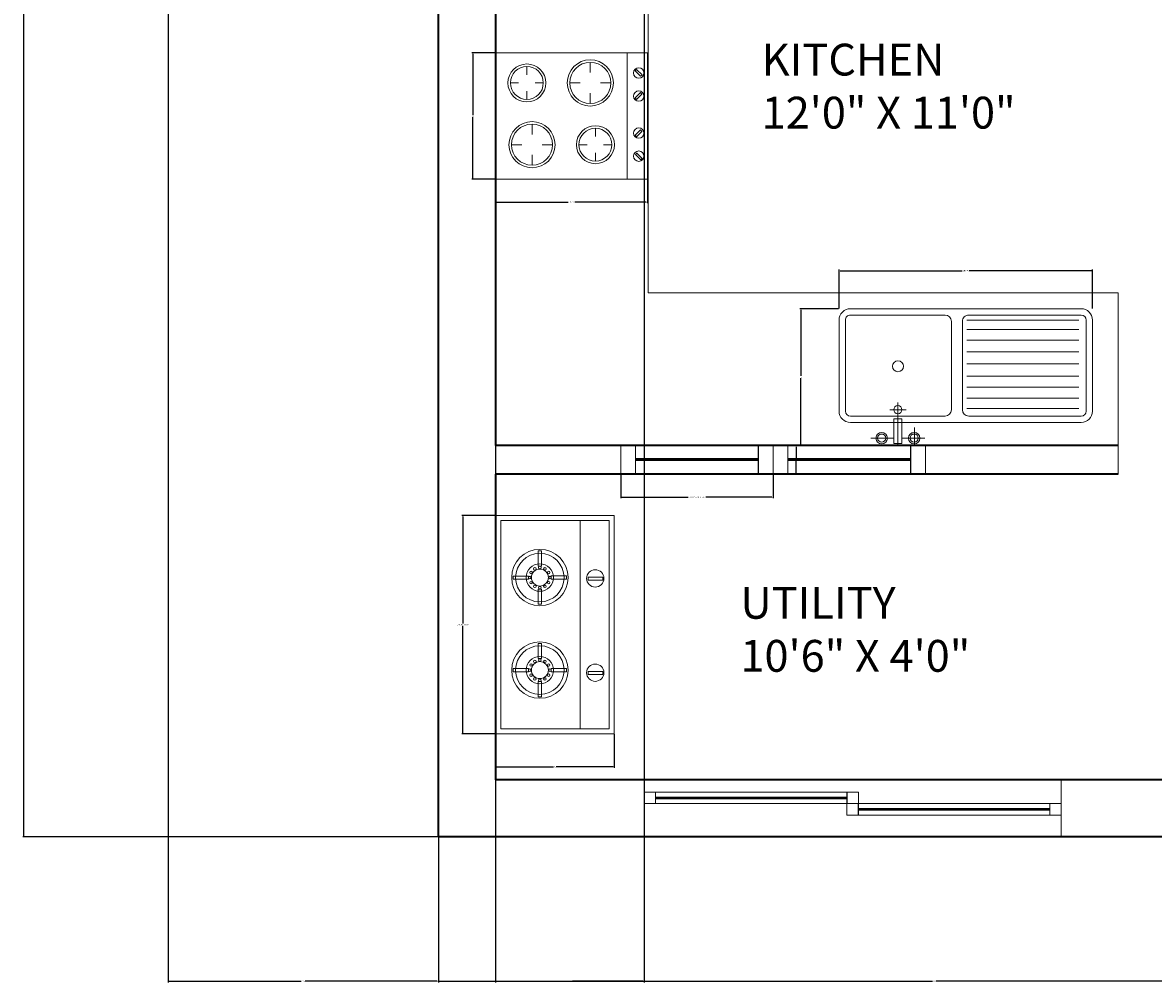
# Model space of a CAD drawing. Units: inches. Extents: x 1723 to 2209, y 1326 to 1810.
# Tile 1 of 6: x 1723 to 1901, y 1326 to 1477. Entities that reach past the tile are written whole.
import ezdxf

# ---------------------------------------------------------------- set-up
doc = ezdxf.new("R2010")
doc.units = ezdxf.units.IN
doc.layers.get('Defpoints').update_dxf_attribs({"color": 255})
for name, color, linetype, lineweight in [('A-ANNO-DIMS', 2, 'Continuous', 18), ('A-AREA-IDEN', 7, 'Continuous', 18), ('A-EQPM', 8, 'Continuous', 13), ('A-FLOR-CASE', 9, 'Continuous', 18), ('A-FLOR-FIXT', 9, 'Continuous', 18), ('A-GLAZ', 4, 'Continuous', 18), ('A-WALL', 7, 'Continuous', 35), ('Sliding Door', 3, 'Continuous', 18)]:
    doc.layers.add(name, color=color, linetype=linetype, lineweight=lineweight)
doc.styles.get("Standard").update_dxf_attribs({"font": 'arial.ttf'})
doc.dimstyles.get("Standard").update_dxf_attribs({"dimtxt": 0.18, "dimasz": 0.18, "dimexe": 0.18, "dimexo": 0.0625, "dimgap": 0.09, "dimtad": 0, "dimtih": 1, "dimtoh": 1, "dimdec": 4, "dimzin": 0, "dimdsep": 46, "dimtxsty": 'Standard', "dimcen": 0.09, "dimadec": 0, "dimazin": 0, "dimtfac": 1, "dimtdec": 4, "dimtofl": 0, "dimtmove": 0, "dimatfit": 3, "dimfxl": 1, "dimtolj": 1, "dimtzin": 0, "dimarcsym": 0})

# ---------------------------------------------------------------- blocks, each defined once
blk = doc.blocks.new('A$C01893FE0')
at = {"ltscale": 1000}
for p, q in [((705.3, 470.5), (705.3, 541.8)), ((770.8, 370.8), (770.8, 541.8)), ((754.6, 512.1), (663.9, 512.1)), ((787, 532.8), (754.6, 532.8)), ((754.6, 435.6), (754.6, 532.8)), ((787, 435.6), (787, 532.8)), ((787, 512.1), (877.6, 512.1)), ((45, 450), (958.9, 450)), ((0, 45), (0, 405)), ((25, 45), (25, 405)), ((45, 425), (490, 425)), ((583.9, 425), (958.9, 425)), ((787, 435.6), (754.6, 435.6)), ((978.9, 405), (978.9, 45)), ((1003.9, 405), (1003.9, 45)), ((53.5, 394.9), (497.4, 394.9)), ((515, 400), (515, 50)), ((558.9, 400), (558.9, 50)), ((803.2, 399.7), (738.4, 399.7)), ((53.5, 353.7), (497.4, 353.7)), ((53.5, 310.3), (497.4, 310.3)), ((53.5, 266.8), (497.4, 266.8)), ((53.5, 218.8), (497.4, 218.8)), ((53.5, 170.8), (497.4, 170.8)), ((53.5, 125), (497.4, 125)), ((53.5, 81.6), (497.4, 81.6)), ((53.5, 45), (497.4, 45)), ((490, 25), (45, 25)), ((958.9, 0), (45, 0)), ((958.9, 25), (583.9, 25))]:
    blk.add_line(p, q, dxfattribs=at)
for centre, radius in [((706.4, 512.1), 22.7), ((706.4, 512.1), 16.2), ((835.2, 512.1), 22.7), ((835.2, 512.1), 16.2), ((771.2, 399.7), 16.2), ((770.4, 227.6), 21.7)]:
    blk.add_circle(centre, radius, dxfattribs=at)
for centre, radius, start, end in [((45, 405), 45, 90, 180), ((958.9, 405), 45, 0, 90), ((45, 405), 20, 90, 180), ((490, 400), 25, 0, 90), ((583.9, 400), 25, 90, 180), ((958.9, 405), 20, 0, 90), ((45, 45), 45, 180, 270), ((45, 45), 20, 180, 270), ((490, 50), 25, 270, 0), ((583.9, 50), 25, 180, 270), ((958.9, 45), 45, 270, 0), ((958.9, 45), 20, 270, 0)]:
    blk.add_arc(centre, radius, start, end, dxfattribs=at)
blk = doc.blocks.new('A$C06E242FC')
for p, q in [((0, 455.6), (0.5, 456.1)), ((0, 455.6), (0, 0.5)), ((838.9, 456.1), (0.5, 456.1)), ((20, 435.6), (20.5, 436.1)), ((20, 435.6), (20, 20.5)), ((818.9, 436.1), (20.5, 436.1)), ((819.4, 435.6), (818.9, 436.1)), ((819.4, 20.5), (819.4, 435.6)), ((838.9, 456.1), (839.4, 455.6)), ((839.4, 0.5), (839.4, 455.6)), ((237.3, 411.5), (237.3, 356.2)), ((248.9, 411.5), (237.3, 411.5)), ((248.9, 356.2), (248.9, 411.5)), ((599.3, 411.5), (610.9, 411.5)), ((599.3, 411.5), (599.3, 356.2)), ((610.9, 356.2), (610.9, 411.5)), ((237.3, 356.2), (248.9, 356.2)), ((599.3, 356.2), (610.9, 356.2)), ((20, 324.4), (819.4, 324.4)), ((232.7, 272.7), (232.7, 214)), ((244.9, 272.7), (232.7, 272.7)), ((244.9, 214), (244.9, 272.7)), ((588.1, 272.7), (588.1, 214)), ((600.3, 272.7), (588.1, 272.7)), ((600.3, 214), (600.3, 272.7)), ((136.3, 176), (136.3, 163.8)), ((194.9, 176), (136.3, 176)), ((194.9, 163.8), (194.9, 176)), ((232.7, 214), (244.9, 214)), ((282.9, 176.3), (282.9, 164.1)), ((341.6, 176.3), (282.9, 176.3)), ((341.6, 164.1), (341.6, 176.3)), ((550.3, 176), (491.7, 176)), ((491.7, 176), (491.7, 163.8)), ((550.3, 163.8), (550.3, 176)), ((588.1, 214), (600.3, 214)), ((638.3, 176.3), (638.3, 164.1)), ((697, 176.3), (638.3, 176.3)), ((697, 164.1), (697, 176.3)), ((136.3, 163.8), (194.9, 163.8)), ((282.9, 164.1), (341.6, 164.1)), ((491.7, 163.8), (550.3, 163.8)), ((638.3, 164.1), (697, 164.1)), ((245.2, 126.1), (233, 126.1)), ((233, 126.1), (233, 67.4)), ((245.2, 67.4), (245.2, 126.1)), ((600.6, 126.1), (588.3, 126.1)), ((588.3, 126.1), (588.3, 67.4)), ((600.6, 67.4), (600.6, 126.1)), ((233, 67.4), (245.2, 67.4)), ((588.3, 67.4), (600.6, 67.4)), ((0, 0.5), (0.5, 0)), ((20, 20.5), (20.5, 20)), ((20.5, 20), (818.9, 20)), ((818.9, 20), (819.4, 20.5)), ((838.9, 0), (839.4, 0.5)), ((0.5, 0), (838.9, 0))]:
    blk.add_line(p, q)
for centre, radius in [((242, 382.9), 33.3), ((604.1, 382.9), 33.3), ((238.9, 170.1), 108.3), ((238.9, 170.1), 93.3), ((594.3, 170.1), 108.3), ((594.3, 170.1), 93.3), ((238.9, 170.1), 52.6), ((594.3, 170.1), 52.6), ((200.1, 170.1), 4.84), ((205.3, 189.5), 4.84), ((238.9, 170.1), 32.6), ((219.5, 203.7), 4.84), ((238.9, 208.9), 4.84), ((258.4, 203.7), 4.84), ((272.6, 189.5), 4.84), ((277.8, 170.1), 4.84), ((555.5, 170.1), 4.84), ((560.7, 189.5), 4.84), ((594.3, 170.1), 32.6), ((574.9, 203.7), 4.84), ((594.3, 208.9), 4.84), ((613.7, 203.7), 4.84), ((628, 189.5), 4.84), ((633.2, 170.1), 4.84), ((205.3, 150.6), 4.84), ((219.5, 136.4), 4.84), ((238.9, 131.2), 4.84), ((258.4, 136.4), 4.84), ((272.6, 150.6), 4.84), ((560.7, 150.6), 4.84), ((574.9, 136.4), 4.84), ((594.3, 131.2), 4.84), ((613.7, 136.4), 4.84), ((628, 150.6), 4.84)]:
    blk.add_circle(centre, radius)
blk = doc.blocks.new('A$C16A60262')
at = {"linetype": 'ByBlock'}
for p, q in [((0, 600), (0, 0)), ((487.7, 600), (0, 600)), ((0, 600), (500, 600)), ((0, 600), (500, 600)), ((500, 600), (500, 0)), ((500, 600), (500, 0)), ((500, 520.4), (0, 520.4)), ((119.4, 455.6), (119.4, 414.9)), ((363.3, 459.6), (363.3, 427.1)), ((38.1, 374.3), (78.8, 374.3)), ((200.7, 374.3), (160.1, 374.3)), ((298.2, 394.6), (330.7, 394.6)), ((363.3, 329.6), (363.3, 362.1)), ((428.3, 394.6), (395.8, 394.6)), ((119.4, 293), (119.4, 333.7)), ((363.3, 225.2), (363.3, 184.6)), ((119.4, 188.6), (119.4, 156.1)), ((282, 143.9), (322.6, 143.9)), ((444.5, 143.9), (403.9, 143.9)), ((54.4, 123.6), (86.9, 123.6)), ((119.4, 58.6), (119.4, 91.1)), ((184.4, 123.6), (151.9, 123.6)), ((363.3, 62.6), (363.3, 103.3)), ((0, 0), (500, 0))]:
    blk.add_line(p, q, dxfattribs=at)
for p, q in [((66.2, 557.5), (87.4, 578.7)), ((71.9, 551.8), (66.2, 557.5)), ((93.1, 573), (71.9, 551.8)), ((87.4, 578.7), (93.1, 573)), ((157.6, 572.5), (163.3, 578.1)), ((178.8, 551.2), (157.6, 572.5)), ((163.3, 578.1), (184.5, 556.9)), ((184.5, 556.9), (178.8, 551.2)), ((305.1, 572.5), (310.8, 578.1)), ((326.3, 551.2), (305.1, 572.5)), ((310.8, 578.1), (332, 556.9)), ((332, 556.9), (326.3, 551.2)), ((396.2, 558.5), (417.4, 579.7)), ((401.9, 552.8), (396.2, 558.5)), ((423.1, 574), (401.9, 552.8)), ((417.4, 579.7), (423.1, 574))]:
    blk.add_line(p, q)
for centre in [(80.1, 565.7), (171.2, 565.7), (317.6, 565.7), (408.7, 565.7)]:
    blk.add_circle(centre, 20.6)
for centre, radius in [((119.4, 374.3), 91.3), ((119.4, 374.3), 81.3), ((363.3, 394.6), 75), ((363.3, 394.6), 65), ((363.3, 143.9), 91.3), ((363.3, 143.9), 81.3), ((119.4, 123.6), 75), ((119.4, 123.6), 65)]:
    blk.add_circle(centre, radius, dxfattribs=at)
blk = doc.blocks.new('A$C7a76cbd6')
at = {"layer": 'Sliding Door'}
for p, q in [((540.4, 283.7, 0), (478.3, 283.7, 0)), ((478.3, 283.7, 0), (540.4, 283.7, 0)), ((540.4, 221.5, 0), (540.4, 283.7, 0)), ((540.4, 283.7, 0), (1585.3, 283.7, 0)), ((540.4, 283.7, 0), (540.4, 221.5, 0)), ((1585.3, 256.6, 0), (540.4, 256.6, 0)), ((540.4, 256.6, 0), (540.4, 248.7, 0)), ((540.4, 252.6, 0), (1584.3, 252.6, 0)), ((540.4, 248.7, 0), (1585.3, 248.7, 0)), ((1584.3, 283.7, 0), (1647.4, 283.7, 0)), ((1584.3, 283.7, 0), (1584.3, 221.5, 0)), ((1647.4, 283.7, 0), (1585.3, 283.7, 0)), ((1585.3, 283.7, 0), (1585.3, 221.5, 0)), ((1585.3, 248.7, 0), (1585.3, 256.6, 0)), ((1647.4, 221.5, 0), (1647.4, 283.7, 0)), ((1647.4, 283.7, 0), (1647.4, 221.5, 0)), ((478.3, 221.5, 0), (540.4, 221.5, 0)), ((478.3, 221.5, 0), (540.4, 221.5, 0)), ((1584.3, 221.5, 0), (540.4, 221.5, 0)), ((1646.4, 221.5, 0), (1584.3, 221.5, 0)), ((1584.3, 221.5, 0), (1584.3, 159.4, 0)), ((1584.3, 221.5, 0), (1647.4, 221.5, 0)), ((1584.3, 221.5, 0), (1647.4, 221.5, 0)), ((1584.3, 221.5, 0), (1584.3, 159.4, 0)), ((1585.3, 221.5, 0), (1647.4, 221.5, 0)), ((1646.4, 159.4, 0), (1646.4, 221.5, 0)), ((1647.4, 221.5, 0), (2691.3, 221.5, 0)), ((1647.4, 221.5, 0), (1647.4, 159.4, 0)), ((2691.3, 194.4, 0), (1647.4, 194.4, 0)), ((1647.4, 194.4, 0), (1647.4, 186.5, 0)), ((1647.4, 190.5, 0), (2690.3, 190.5, 0)), ((1647.4, 186.5, 0), (2691.3, 186.5, 0)), ((2690.3, 221.5, 0), (2753.4, 221.5, 0)), ((2690.3, 221.5, 0), (2690.3, 159.4, 0)), ((2753.4, 221.5, 0), (2691.3, 221.5, 0)), ((2691.3, 221.5, 0), (2691.3, 159.4, 0)), ((2691.3, 186.5, 0), (2691.3, 194.4, 0)), ((1584.3, 159.4, 0), (1646.4, 159.4, 0)), ((1584.3, 159.4, 0), (1647.4, 159.4, 0)), ((2691.3, 159.4, 0), (1646.4, 159.4, 0)), ((2690.3, 159.4, 0), (2753.4, 159.4, 0)), ((2691.3, 159.4, 0), (2753.4, 159.4, 0))]:
    blk.add_line(p, q, dxfattribs=at)
blk = doc.blocks.new('WINDOW-UTILITY-SASH')
for p, q in [((0, 4.5), (0, 0)), ((0, 4.5), (0, 0)), ((0, 4.5), (2.33, 4.5)), ((2.3, 0), (2.3, 4.5)), ((23.95, 4.5), (2.3, 4.5)), ((2.33, 4.5), (2.33, 0)), ((21.62, 4.5), (21.62, 0)), ((21.62, 4.5), (23.95, 4.5)), ((21.66, 4.5), (21.66, 0)), ((23.95, 4.5), (23.95, 0)), ((21.62, 2.47), (2.33, 2.47)), ((2.33, 2.33), (21.62, 2.33)), ((2.33, 2.18), (21.62, 2.18)), ((0, 0), (2.3, 0)), ((0, 0), (2.33, 0)), ((23.95, 0), (2.3, 0)), ((2.33, 1.29), (2.33, 1)), ((21.62, 0), (23.95, 0)), ((21.66, 1), (21.66, 1.29)), ((21.66, 0), (23.95, 0))]:
    blk.add_line(p, q)
blk = doc.blocks.new('*D77')
at = {"layer": 'A-ANNO-DIMS', "color": 0, "lineweight": -2, "transparency": 16777216}
for p, q in [((1816.79, 1405.63), (1816.79, 1401.92)), ((1840.74, 1405.63), (1840.74, 1401.92)), ((1816.97, 1402.1), (1827.36, 1402.1)), ((1840.56, 1402.1), (1830.17, 1402.1))]:
    blk.add_line(p, q, dxfattribs=at)
at = {"layer": 'A-ANNO-DIMS', "color": 0, "transparency": 16777216}
for points in [[(1816.97, 1402.13), (1816.97, 1402.07), (1816.79, 1402.1)], [(1840.56, 1402.13), (1840.56, 1402.07), (1840.74, 1402.1)]]:
    blk.add_solid(points, dxfattribs=at)
at = {"layer": 'Defpoints', "color": 0, "transparency": 16777216}
for p in [(1816.79, 1405.69), (1840.74, 1405.69), (1840.74, 1402.1)]:
    blk.add_point(p, dxfattribs=at)
at = {"layer": 'A-ANNO-DIMS', "color": 0, "transparency": 16777216, "insert": (1828.76, 1402.1), "char_height": 0.18, "attachment_point": 5}
blk.add_mtext('\\A1;UTILITY SASH 24 TYP.', dxfattribs=at)
blk = doc.blocks.new('*D78')
at = {"layer": 'A-ANNO-DIMS', "color": 0, "lineweight": -2, "transparency": 16777216}
for p, q in [((1840.8, 1410.19), (1844.52, 1410.19)), ((1844.34, 1410.01), (1844.34, 1408.12)), ((1844.34, 1405.87), (1844.34, 1407.76)), ((1840.8, 1405.69), (1844.52, 1405.69))]:
    blk.add_line(p, q, dxfattribs=at)
at = {"layer": 'A-ANNO-DIMS', "color": 0, "transparency": 16777216}
for points in [[(1844.31, 1410.01), (1844.37, 1410.01), (1844.34, 1410.19)], [(1844.31, 1405.87), (1844.37, 1405.87), (1844.34, 1405.69)]]:
    blk.add_solid(points, dxfattribs=at)
at = {"layer": 'Defpoints', "color": 0, "transparency": 16777216}
for p in [(1840.74, 1410.19), (1844.34, 1410.19), (1840.74, 1405.69)]:
    blk.add_point(p, dxfattribs=at)
at = {"layer": 'A-ANNO-DIMS', "color": 0, "transparency": 16777216, "insert": (1844.34, 1407.94), "char_height": 0.18, "attachment_point": 5}
blk.add_mtext('\\A1;5 TYP.', dxfattribs=at)
blk = doc.blocks.new('*D79')
at = {"layer": 'A-ANNO-DIMS', "color": 0, "lineweight": -2, "transparency": 16777216}
for p, q in [((1851.1, 1431.76), (1851.1, 1437.86)), ((1851.28, 1437.68), (1870.49, 1437.68)), ((1890.78, 1437.68), (1871.58, 1437.68)), ((1890.96, 1431.76), (1890.96, 1437.86))]:
    blk.add_line(p, q, dxfattribs=at)
at = {"layer": 'A-ANNO-DIMS', "color": 0, "transparency": 16777216}
for points in [[(1851.28, 1437.71), (1851.28, 1437.65), (1851.1, 1437.68)], [(1890.78, 1437.71), (1890.78, 1437.65), (1890.96, 1437.68)]]:
    blk.add_solid(points, dxfattribs=at)
at = {"layer": 'Defpoints', "color": 0, "transparency": 16777216}
for p in [(1851.1, 1437.68), (1851.1, 1431.7), (1890.96, 1431.7)]:
    blk.add_point(p, dxfattribs=at)
at = {"layer": 'A-ANNO-DIMS', "color": 0, "transparency": 16777216, "insert": (1871.03, 1437.68), "char_height": 0.18, "attachment_point": 5}
blk.add_mtext('\\A1;SINK 40', dxfattribs=at)
blk = doc.blocks.new('*D80')
at = {"layer": 'A-ANNO-DIMS', "color": 0, "lineweight": -2, "transparency": 16777216}
for p, q in [((1851.04, 1431.7), (1844.94, 1431.7)), ((1845.12, 1431.52), (1845.12, 1421.13)), ((1845.12, 1410.37), (1845.12, 1420.77)), ((1851.04, 1410.19), (1844.94, 1410.19))]:
    blk.add_line(p, q, dxfattribs=at)
at = {"layer": 'A-ANNO-DIMS', "color": 0, "transparency": 16777216}
for points in [[(1845.09, 1431.52), (1845.15, 1431.52), (1845.12, 1431.7)], [(1845.09, 1410.37), (1845.15, 1410.37), (1845.12, 1410.19)]]:
    blk.add_solid(points, dxfattribs=at)
at = {"layer": 'Defpoints', "color": 0, "transparency": 16777216}
for p in [(1851.1, 1431.7), (1845.12, 1410.19), (1851.1, 1410.19)]:
    blk.add_point(p, dxfattribs=at)
at = {"layer": 'A-ANNO-DIMS', "color": 0, "transparency": 16777216, "insert": (1845.12, 1420.95), "char_height": 0.18, "attachment_point": 5}
blk.add_mtext('\\A1;22', dxfattribs=at)
blk = doc.blocks.new('*D81')
at = {"layer": 'A-ANNO-DIMS', "color": 0, "lineweight": -2, "transparency": 16777216}
for p, q in [((1797.04, 1399.23), (1791.77, 1399.23)), ((1791.95, 1399.05), (1791.95, 1382.24)), ((1791.95, 1365.06), (1791.95, 1381.87)), ((1797.04, 1364.88), (1791.77, 1364.88))]:
    blk.add_line(p, q, dxfattribs=at)
at = {"layer": 'A-ANNO-DIMS', "color": 0, "transparency": 16777216}
for points in [[(1791.92, 1399.05), (1791.98, 1399.05), (1791.95, 1399.23)], [(1791.92, 1365.06), (1791.98, 1365.06), (1791.95, 1364.88)]]:
    blk.add_solid(points, dxfattribs=at)
at = {"layer": 'Defpoints', "color": 0, "transparency": 16777216}
for p in [(1797.1, 1399.23), (1791.95, 1364.88), (1797.1, 1364.88)]:
    blk.add_point(p, dxfattribs=at)
at = {"layer": 'A-ANNO-DIMS', "color": 0, "transparency": 16777216, "insert": (1791.95, 1382.05), "char_height": 0.18, "attachment_point": 5}
blk.add_mtext('\\A1;UTILITY HOB 34', dxfattribs=at)
blk = doc.blocks.new('*D82')
at = {"layer": 'A-ANNO-DIMS', "color": 0, "lineweight": -2, "transparency": 16777216}
for p, q in [((1797.1, 1364.82), (1797.1, 1359.55)), ((1815.77, 1364.82), (1815.77, 1359.55)), ((1797.28, 1359.73), (1806.22, 1359.73)), ((1815.59, 1359.73), (1806.64, 1359.73))]:
    blk.add_line(p, q, dxfattribs=at)
at = {"layer": 'A-ANNO-DIMS', "color": 0, "transparency": 16777216}
for points in [[(1797.28, 1359.76), (1797.28, 1359.7), (1797.1, 1359.73)], [(1815.59, 1359.76), (1815.59, 1359.7), (1815.77, 1359.73)]]:
    blk.add_solid(points, dxfattribs=at)
at = {"layer": 'Defpoints', "color": 0, "transparency": 16777216}
for p in [(1797.1, 1364.88), (1815.77, 1364.88), (1815.77, 1359.73)]:
    blk.add_point(p, dxfattribs=at)
at = {"layer": 'A-ANNO-DIMS', "color": 0, "transparency": 16777216, "insert": (1806.43, 1359.73), "char_height": 0.18, "attachment_point": 5}
blk.add_mtext('\\A1;19', dxfattribs=at)
blk = doc.blocks.new('*D83')
at = {"layer": 'A-ANNO-DIMS', "color": 0, "lineweight": -2, "transparency": 16777216}
for p, q in [((1797.1, 1451.98), (1797.1, 1448.28)), ((1820.97, 1451.98), (1820.97, 1448.28)), ((1797.28, 1448.46), (1808.52, 1448.46)), ((1820.79, 1448.46), (1809.56, 1448.46))]:
    blk.add_line(p, q, dxfattribs=at)
at = {"layer": 'A-ANNO-DIMS', "color": 0, "transparency": 16777216}
for points in [[(1797.28, 1448.49), (1797.28, 1448.43), (1797.1, 1448.46)], [(1820.79, 1448.49), (1820.79, 1448.43), (1820.97, 1448.46)]]:
    blk.add_solid(points, dxfattribs=at)
at = {"layer": 'Defpoints', "color": 0, "transparency": 16777216}
for p in [(1797.1, 1452.04), (1820.97, 1452.04), (1820.97, 1448.46)]:
    blk.add_point(p, dxfattribs=at)
at = {"layer": 'A-ANNO-DIMS', "color": 0, "transparency": 16777216, "insert": (1809.04, 1448.46), "char_height": 0.18, "attachment_point": 5}
blk.add_mtext('\\A1;HOB 24', dxfattribs=at)
blk = doc.blocks.new('*D84')
at = {"layer": 'A-ANNO-DIMS', "color": 0, "lineweight": -2, "transparency": 16777216}
for p, q in [((1797.04, 1471.93), (1793.34, 1471.93)), ((1793.52, 1471.75), (1793.52, 1462.17)), ((1793.52, 1452.22), (1793.52, 1461.8)), ((1797.04, 1452.04), (1793.34, 1452.04))]:
    blk.add_line(p, q, dxfattribs=at)
at = {"layer": 'A-ANNO-DIMS', "color": 0, "transparency": 16777216}
for points in [[(1793.49, 1471.75), (1793.55, 1471.75), (1793.52, 1471.93)], [(1793.49, 1452.22), (1793.55, 1452.22), (1793.52, 1452.04)]]:
    blk.add_solid(points, dxfattribs=at)
at = {"layer": 'Defpoints', "color": 0, "transparency": 16777216}
for p in [(1797.1, 1471.93), (1793.52, 1452.04), (1797.1, 1452.04)]:
    blk.add_point(p, dxfattribs=at)
at = {"layer": 'A-ANNO-DIMS', "color": 0, "transparency": 16777216, "insert": (1793.52, 1461.99), "char_height": 0.18, "attachment_point": 5}
blk.add_mtext('\\A1;20', dxfattribs=at)
blk = doc.blocks.new('*D94')
at = {"layer": 'A-ANNO-DIMS', "color": 0, "lineweight": -2, "transparency": 16777216}
for p, q in [((1788.04, 1786.69), (1722.75, 1786.69)), ((1722.93, 1786.51), (1722.93, 1567.87)), ((1722.93, 1348.87), (1722.93, 1567.51)), ((1788.04, 1348.69), (1722.75, 1348.69))]:
    blk.add_line(p, q, dxfattribs=at)
at = {"layer": 'A-ANNO-DIMS', "color": 0, "transparency": 16777216}
for points in [[(1722.9, 1786.51), (1722.96, 1786.51), (1722.93, 1786.69)], [(1722.9, 1348.87), (1722.96, 1348.87), (1722.93, 1348.69)]]:
    blk.add_solid(points, dxfattribs=at)
at = {"layer": 'Defpoints', "color": 0, "transparency": 16777216}
for p in [(1722.93, 1786.69), (1788.1, 1786.69), (1788.1, 1348.69)]:
    blk.add_point(p, dxfattribs=at)
at = {"layer": 'A-ANNO-DIMS', "color": 0, "transparency": 16777216, "insert": (1722.93, 1567.69), "char_height": 0.18, "attachment_point": 5}
blk.add_mtext('\\A1;438', dxfattribs=at)
blk = doc.blocks.new('*D95')
at = {"layer": 'A-ANNO-DIMS', "color": 0, "lineweight": -2, "transparency": 16777216}
for p, q in [((1745.6, 1487.63), (1745.6, 1325.84)), ((1788.1, 1348.63), (1788.1, 1325.84)), ((1745.78, 1326.02), (1766.53, 1326.02)), ((1787.92, 1326.02), (1767.18, 1326.02))]:
    blk.add_line(p, q, dxfattribs=at)
at = {"layer": 'A-ANNO-DIMS', "color": 0, "transparency": 16777216}
for points in [[(1745.78, 1326.05), (1745.78, 1325.99), (1745.6, 1326.02)], [(1787.92, 1326.05), (1787.92, 1325.99), (1788.1, 1326.02)]]:
    blk.add_solid(points, dxfattribs=at)
at = {"layer": 'Defpoints', "color": 0, "transparency": 16777216}
for p in [(1745.6, 1487.69), (1788.1, 1348.69), (1788.1, 1326.02)]:
    blk.add_point(p, dxfattribs=at)
at = {"layer": 'A-ANNO-DIMS', "color": 0, "transparency": 16777216, "insert": (1766.85, 1326.02), "char_height": 0.18, "attachment_point": 5}
blk.add_mtext('\\A1;42.5', dxfattribs=at)
blk = doc.blocks.new('*D96')
at = {"layer": 'A-ANNO-DIMS', "color": 0, "lineweight": -2, "transparency": 16777216}
for p, q in [((1944.1, 1357.63), (1944.1, 1325.84)), ((1788.1, 1348.63), (1788.1, 1325.84)), ((1788.28, 1326.02), (1865.82, 1326.02)), ((1943.92, 1326.02), (1866.38, 1326.02))]:
    blk.add_line(p, q, dxfattribs=at)
at = {"layer": 'A-ANNO-DIMS', "color": 0, "transparency": 16777216}
for points in [[(1788.28, 1326.05), (1788.28, 1325.99), (1788.1, 1326.02)], [(1943.92, 1326.05), (1943.92, 1325.99), (1944.1, 1326.02)]]:
    blk.add_solid(points, dxfattribs=at)
at = {"layer": 'Defpoints', "color": 0, "transparency": 16777216}
for p in [(1944.1, 1357.69), (1788.1, 1348.69), (1944.1, 1326.02)]:
    blk.add_point(p, dxfattribs=at)
at = {"layer": 'A-ANNO-DIMS', "color": 0, "transparency": 16777216, "insert": (1866.1, 1326.02), "char_height": 0.18, "attachment_point": 5}
blk.add_mtext('\\A1;156', dxfattribs=at)
blk = doc.blocks.new('*D114')
at = {"layer": 'A-ANNO-DIMS', "color": 0, "lineweight": -2, "transparency": 16777216}
for p, q in [((1797.1, 1777.63), (1797.1, 1325.84)), ((1820.45, 1777.63), (1820.45, 1325.84)), ((1797.28, 1326.02), (1808.38, 1326.02)), ((1820.27, 1326.02), (1809.17, 1326.02))]:
    blk.add_line(p, q, dxfattribs=at)
at = {"layer": 'A-ANNO-DIMS', "color": 0, "transparency": 16777216}
for points in [[(1797.28, 1326.05), (1797.28, 1325.99), (1797.1, 1326.02)], [(1820.27, 1326.05), (1820.27, 1325.99), (1820.45, 1326.02)]]:
    blk.add_solid(points, dxfattribs=at)
at = {"layer": 'Defpoints', "color": 0, "transparency": 16777216}
for p in [(1797.1, 1777.69), (1820.45, 1777.69), (1820.45, 1326.02)]:
    blk.add_point(p, dxfattribs=at)
at = {"layer": 'A-ANNO-DIMS', "color": 0, "transparency": 16777216, "insert": (1808.78, 1326.02), "char_height": 0.18, "attachment_point": 5}
blk.add_mtext('\\A1;23.35', dxfattribs=at)

msp = doc.modelspace()

# ---------------------------------------------------------------- linework, layer by layer
at = {"layer": 'A-FLOR-CASE'}
for p, q in [((1821.1032, 1501.6915), (1821.1032, 1434.1915)), ((1894.9851, 1434.1915), (1821.1032, 1434.1915)), ((1894.9851, 1434.1915), (1894.9851, 1405.6915))]:
    msp.add_line(p, q, dxfattribs=at)
at = {"layer": 'A-GLAZ'}
for p, q in [((1820.4509, 1357.6915), (1820.4509, 1348.6915)), ((1886.0318, 1357.6915), (1886.0318, 1348.6915))]:
    msp.add_line(p, q, dxfattribs=at)
at = {"layer": 'A-WALL'}
for p, q in [((1797.1032, 1501.6915), (1797.1032, 1410.1915)), ((1894.9851, 1410.1915), (1797.1032, 1410.1915)), ((1797.1032, 1405.6915), (1797.1032, 1357.6915)), ((1894.9851, 1405.6915), (1797.1032, 1405.6915)), ((1939.6032, 1357.6915), (1797.1032, 1357.6915))]:
    msp.add_line(p, q, dxfattribs=at)
msp.add_lwpolyline([(2185.6032, 1576.485), (2185.6032, 1348.6915), (1788.1032, 1348.6915), (1788.1032, 1506.1915)], dxfattribs=at)

# ---------------------------------------------------------------- block references
at = {"layer": 'A-EQPM', "rotation": 270}
for name, p, xscale, yscale, zscale in [('A$C16A60262', (1797.1032, 1471.9319), 0.039781326106008, 0.039781326106008, 0.039781326106008), ('A$C06E242FC', (1797.1032, 1399.2263), 0.0409160479911132, 0.0409160479911132, 0.0409160479911132)]:
    msp.add_blockref(name, p, dxfattribs=dict(at, xscale=xscale, yscale=yscale, zscale=zscale))
at = {"layer": 'A-FLOR-FIXT', "xscale": 0.0397036692982852, "yscale": 0.0397036692982852, "zscale": 0.0397036692982852, "rotation": 180}
msp.add_blockref('A$C01893FE0', (1890.9619, 1431.7022), dxfattribs=at)
at = {"layer": 'A-GLAZ'}
msp.add_blockref('WINDOW-UTILITY-SASH', (1816.7873, 1405.6915), dxfattribs=at)
at = {"layer": 'A-GLAZ', "extrusion": (0, 0, -1), "zscale": -1}
msp.add_blockref('WINDOW-UTILITY-SASH', (-1864.697, 1405.6915), dxfattribs=at)
at = {"layer": 'A-GLAZ', "xscale": 0.0288245099661422, "yscale": 0.0288245099661422, "zscale": 0.0288245099661422, "rotation": 180}
msp.add_blockref('A$C7a76cbd6', (1899.8174, 1360.309), dxfattribs=at)

# ---------------------------------------------------------------- texts
at = {"layer": 'A-AREA-IDEN', "char_height": 5, "attachment_point": 1}
for s, width, insert in [('KITCHEN\\P12\'0" X 11\'0"', 63.696937, (1838.9286, 1473.3486)), ('UTILITY\\P10\'6" X 4\'0"', 48.552212, (1835.5941, 1387.9869))]:
    msp.add_mtext_dynamic_manual_height_columns(s, width=width, gutter_width=12.5, heights=[0], dxfattribs=dict(at, insert=insert))

# ---------------------------------------------------------------- dimensions: what is measured, and where the dimension line sits
at = {"layer": 'A-ANNO-DIMS'}
for base, p1, p2, angle, picture, middle in [((1722.9332, 1786.6915), (1788.1032, 1348.6915), (1788.1032, 1786.6915), 90, '*D94', (1722.9332, 1567.6915)), ((1793.5228, 1452.0413), (1797.1032, 1471.9319), (1797.1032, 1452.0413), 270, '*D84', (1793.5228, 1461.9866)), ((1845.1247, 1410.1915), (1851.1035, 1431.7022), (1851.1035, 1410.1915), 270, '*D80', (1845.1247, 1420.9468))]:
    dim = msp.add_linear_dim(base=base, p1=p1, p2=p2, angle=angle, dimstyle='Standard', override={"dimdec": 0, "dimlfac": 1, "dimrnd": 0, "dimzin": 0, "dimdsep": 46, "dimlunit": 2}, dxfattribs=at)
    dim.commit()
    dim.dimension.update_dxf_attribs({"geometry": picture, "text_midpoint": middle})
for base, p1, p2, override, picture, middle in [((1820.4509, 1326.0215), (1797.1032, 1777.6915), (1820.4509, 1777.6915), {"dimdec": 2, "dimlfac": 1, "dimrnd": 0, "dimzin": 0, "dimdsep": 46, "dimlunit": 2}, '*D114', (1808.777, 1326.0215)), ((1788.1032, 1326.0215), (1745.6032, 1487.6915), (1788.1032, 1348.6915), {"dimdec": 1, "dimlfac": 1, "dimrnd": 0, "dimzin": 0, "dimdsep": 46, "dimlunit": 2}, '*D95', (1766.8532, 1326.0215)), ((1815.7655, 1359.7298), (1797.1032, 1364.8815), (1815.7655, 1364.8815), {"dimdec": 0, "dimlfac": 1, "dimrnd": 0, "dimzin": 0, "dimdsep": 46, "dimlunit": 2}, '*D82', (1806.4343, 1359.7298)), ((1944.1032, 1326.0215), (1788.1032, 1348.6915), (1944.1032, 1357.6915), {"dimdec": 0, "dimlfac": 1, "dimrnd": 0, "dimzin": 0, "dimdsep": 46, "dimlunit": 2}, '*D96', (1866.1032, 1326.0215))]:
    dim = msp.add_linear_dim(base=base, p1=p1, p2=p2, dimstyle='Standard', override=override, dxfattribs=at)
    dim.commit()
    dim.dimension.update_dxf_attribs({"geometry": picture, "text_midpoint": middle})
for base, p1, p2, text, picture, middle in [((1820.9719, 1448.461), (1797.1032, 1452.0413), (1820.9719, 1452.0413), 'HOB <>', '*D83', (1809.0375, 1448.461)), ((1840.7422, 1402.0983), (1816.7873, 1405.6915), (1840.7422, 1405.6915), 'UTILITY SASH <> TYP.', '*D77', (1828.7647, 1402.0983))]:
    dim = msp.add_linear_dim(base=base, p1=p1, p2=p2, text=text, dimstyle='Standard', override={"dimdec": 0, "dimlfac": 1, "dimrnd": 0, "dimzin": 0, "dimdsep": 46, "dimlunit": 2}, dxfattribs=at)
    dim.commit()
    dim.dimension.update_dxf_attribs({"geometry": picture, "text_midpoint": middle})
for base, p1, p2, angle, text, picture, middle in [((1851.1035, 1437.6809), (1890.9619, 1431.7022), (1851.1035, 1431.7022), 180, 'SINK <>', '*D79', (1871.0327, 1437.6809)), ((1844.3353787129, 1410.1915089226), (1840.7421529115, 1405.6915089226), (1840.7421529115, 1410.1915089226), 90, '<> TYP.', '*D78', (1844.3353787129, 1407.9415089226)), ((1791.9514, 1364.8815), (1797.1032, 1399.2263), (1797.1032, 1364.8815), 270, 'UTILITY HOB <>', '*D81', (1791.9514, 1382.0539))]:
    dim = msp.add_linear_dim(base=base, p1=p1, p2=p2, angle=angle, text=text, dimstyle='Standard', override={"dimdec": 0, "dimlfac": 1, "dimrnd": 0, "dimzin": 0, "dimdsep": 46, "dimlunit": 2}, dxfattribs=at)
    dim.commit()
    dim.dimension.update_dxf_attribs({"geometry": picture, "text_midpoint": middle})

doc.saveas('drawing.dxf')
